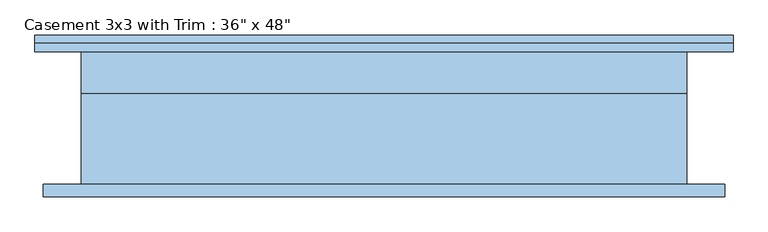
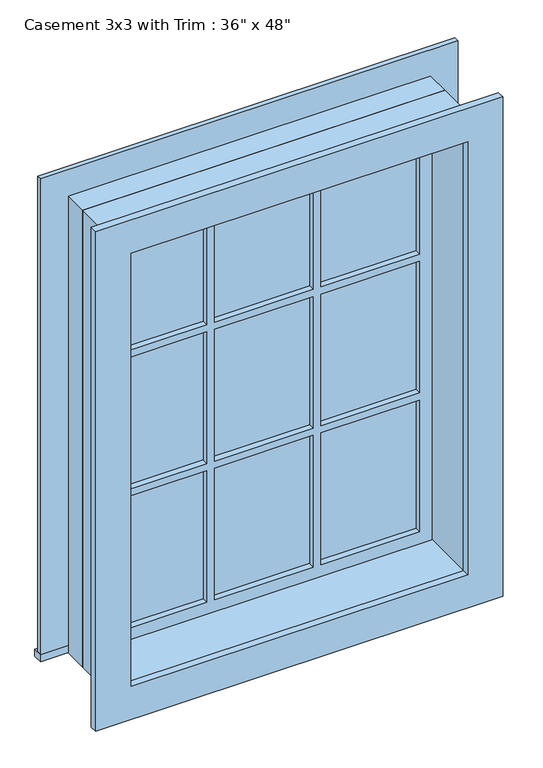
"""IFC4 building model written with IfcOpenShell, lengths in millimetres: window geometry."""

from ifc_helpers import new_model, si_unit, frame, origin, place, context, project, spatial, polyline, outline, extrude, source, transform, mapped, element, save


def window_ddc5d35f(model_context):
    return source(origin(), model_context, "Body", "SweptSolid", [
        extrude(outline(polyline([(-527.05, 125.4), (527.05, 125.4), (527.05, 100.0), (-527.05, 100.0), (-527.05, 125.4)])), frame((0.0, 0.0, 914.4), z_axis=(0.0, 0.0, 1.0), x_axis=(1.0, 0.0, 0.0)), (0.0, 0.0, 1.0), 19.05),
        extrude(outline(polyline([(2114.55, -438.15), (2114.55, 438.15), (933.45, 438.15), (933.45, 527.05), (2203.45, 527.05), (2203.45, -527.05), (933.45, -527.05), (933.45, -438.15), (2114.55, -438.15)])), frame((0.0, 100.0, 0.0), z_axis=(0.0, 1.0, 0.0), x_axis=(0.0, 0.0, 1.0)), (0.0, 0.0, 1.0), 12.7),
        extrude(outline(polyline([(143.9333333, 65.075), (393.7, 65.075), (393.7, 52.375), (143.9333333, 52.375), (143.9333333, 65.075)])), frame((0.0, 0.0, 1718.7333333), z_axis=(0.0, 0.0, 1.0), x_axis=(1.0, 0.0, 0.0)), (0.0, 0.0, 1.0), 351.3666667),
        extrude(outline(polyline([(-124.8833333, 65.075), (124.8833333, 65.075), (124.8833333, 52.375), (-124.8833333, 52.375), (-124.8833333, 65.075)])), frame((0.0, 0.0, 1718.7333333), z_axis=(0.0, 0.0, 1.0), x_axis=(1.0, 0.0, 0.0)), (0.0, 0.0, 1.0), 351.3666667),
        extrude(outline(polyline([(-393.7, 65.075), (-143.9333333, 65.075), (-143.9333333, 52.375), (-393.7, 52.375), (-393.7, 65.075)])), frame((0.0, 0.0, 1718.7333333), z_axis=(0.0, 0.0, 1.0), x_axis=(1.0, 0.0, 0.0)), (0.0, 0.0, 1.0), 351.3666667),
        extrude(outline(polyline([(-393.7, 65.075), (-143.9333333, 65.075), (-143.9333333, 52.375), (-393.7, 52.375), (-393.7, 65.075)])), frame((0.0, 0.0, 1348.3166667), z_axis=(0.0, 0.0, 1.0), x_axis=(1.0, 0.0, 0.0)), (0.0, 0.0, 1.0), 351.3666667),
        extrude(outline(polyline([(-124.8833333, 65.075), (124.8833333, 65.075), (124.8833333, 52.375), (-124.8833333, 52.375), (-124.8833333, 65.075)])), frame((0.0, 0.0, 1348.3166667), z_axis=(0.0, 0.0, 1.0), x_axis=(1.0, 0.0, 0.0)), (0.0, 0.0, 1.0), 351.3666667),
        extrude(outline(polyline([(143.9333333, 65.075), (393.7, 65.075), (393.7, 52.375), (143.9333333, 52.375), (143.9333333, 65.075)])), frame((0.0, 0.0, 1348.3166667), z_axis=(0.0, 0.0, 1.0), x_axis=(1.0, 0.0, 0.0)), (0.0, 0.0, 1.0), 351.3666667),
        extrude(outline(polyline([(143.9333333, 65.075), (393.7, 65.075), (393.7, 52.375), (143.9333333, 52.375), (143.9333333, 65.075)])), frame((0.0, 0.0, 977.9), z_axis=(0.0, 0.0, 1.0), x_axis=(1.0, 0.0, 0.0)), (0.0, 0.0, 1.0), 351.3666667),
        extrude(outline(polyline([(-124.8833333, 65.075), (124.8833333, 65.075), (124.8833333, 52.375), (-124.8833333, 52.375), (-124.8833333, 65.075)])), frame((0.0, 0.0, 977.9), z_axis=(0.0, 0.0, 1.0), x_axis=(1.0, 0.0, 0.0)), (0.0, 0.0, 1.0), 351.3666667),
        extrude(outline(polyline([(-393.7, 65.075), (-143.9333333, 65.075), (-143.9333333, 52.375), (-393.7, 52.375), (-393.7, 65.075)])), frame((0.0, 0.0, 977.9), z_axis=(0.0, 0.0, 1.0), x_axis=(1.0, 0.0, 0.0)), (0.0, 0.0, 1.0), 351.3666667),
        extrude(outline(polyline([(2190.75, 514.35), (2190.75, -514.35), (857.25, -514.35), (857.25, 514.35), (2190.75, 514.35)]), holes=[polyline([(2101.85, 425.45), (946.15, 425.45), (946.15, -425.45), (2101.85, -425.45), (2101.85, 425.45)])]), frame((0.0, -119.05, 0.0), z_axis=(0.0, 1.0, 0.0), x_axis=(0.0, 0.0, 1.0)), (0.0, 0.0, 1.0), 19.05),
        extrude(outline(polyline([(2114.55, -438.15), (933.45, -438.15), (933.45, 438.15), (2114.55, 438.15), (2114.55, -438.15)]), holes=[polyline([(2070.1, -143.9333333), (1718.7333333, -143.9333333), (1718.7333333, -393.7), (2070.1, -393.7), (2070.1, -143.9333333)]), polyline([(1699.6833333, -143.9333333), (1348.3166667, -143.9333333), (1348.3166667, -393.7), (1699.6833333, -393.7), (1699.6833333, -143.9333333)]), polyline([(1329.2666667, -143.9333333), (977.9, -143.9333333), (977.9, -393.7), (1329.2666667, -393.7), (1329.2666667, -143.9333333)]), polyline([(2070.1, 124.8833333), (1718.7333333, 124.8833333), (1718.7333333, -124.8833333), (2070.1, -124.8833333), (2070.1, 124.8833333)]), polyline([(1699.6833333, 124.8833333), (1348.3166667, 124.8833333), (1348.3166667, -124.8833333), (1699.6833333, -124.8833333), (1699.6833333, 124.8833333)]), polyline([(1329.2666667, 124.8833333), (977.9, 124.8833333), (977.9, -124.8833333), (1329.2666667, -124.8833333), (1329.2666667, 124.8833333)]), polyline([(2070.1, 393.7), (1718.7333333, 393.7), (1718.7333333, 143.9333333), (2070.1, 143.9333333), (2070.1, 393.7)]), polyline([(1699.6833333, 393.7), (1348.3166667, 393.7), (1348.3166667, 143.9333333), (1699.6833333, 143.9333333), (1699.6833333, 393.7)]), polyline([(1329.2666667, 393.7), (977.9, 393.7), (977.9, 143.9333333), (1329.2666667, 143.9333333), (1329.2666667, 393.7)])]), frame((0.0, 36.5, 0.0), z_axis=(0.0, 1.0, 0.0), x_axis=(0.0, 0.0, 1.0)), (0.0, 0.0, 1.0), 44.45),
        extrude(outline(polyline([(2133.6, -457.2), (914.4, -457.2), (914.4, 457.2), (2133.6, 457.2), (2133.6, -457.2)]), holes=[polyline([(2101.85, -425.45), (2101.85, 425.45), (946.15, 425.45), (946.15, -425.45), (2101.85, -425.45)])]), frame((0.0, -100.0, 0.0), z_axis=(0.0, 1.0, 0.0), x_axis=(0.0, 0.0, 1.0)), (0.0, 0.0, 1.0), 136.5),
        extrude(outline(polyline([(2133.6, 457.2), (2133.6, -457.2), (914.4, -457.2), (914.4, 457.2), (2133.6, 457.2)]), holes=[polyline([(2114.55, 438.15), (933.45, 438.15), (933.45, -438.15), (2114.55, -438.15), (2114.55, 438.15)])]), frame((0.0, 36.5, 0.0), z_axis=(0.0, 1.0, 0.0), x_axis=(0.0, 0.0, 1.0)), (0.0, 0.0, 1.0), 63.5),
    ])


if __name__ == "__main__":
    model = new_model("IFC4")
    model_context = context("Model", 3, world=origin())
    ifc_project = project(units=[si_unit("LENGTHUNIT", "METRE", prefix="MILLI")], contexts=[model_context])
    site = spatial("IfcSite", under=ifc_project)
    building = spatial("IfcBuilding", under=site)
    placement = place(None, origin())
    window_shape = window_ddc5d35f(model_context)
    element("IfcWindow", 1, ObjectType="Casement 3x3 with Trim : 36\" x 48\"", at=placement, inside=building, context=model_context, shape_type="MappedRepresentation", body=[
        mapped(window_shape, transform((0.0, 0.0, 0.0), x_axis=(1.0, 0.0, 0.0), y_axis=(0.0, 1.0, 0.0), z_axis=(0.0, 0.0, 1.0))),
    ])
    save(model, "model.ifc")

# Revit data of these elements
# Type "Casement 3x3 with Trim : 36\" x 48\""
#   Type Mark = "19"
#   Construction Type Id = "GSP4R"
#   Assembly Code = "B2020100"
#   Analytic Construction = "1/8 in Pilkington single glazing"
#   Visual Light Transmittance = 0.9
#   Solar Heat Gain Coefficient = 0.78
#   Heat Transfer Coefficient (U) = 3.6886 W/(m²·K)
#   Height = 4' - 0"
#   Default Sill Height = 3' - 0"
#   Trim Projection - Ext. = 0' - 0 1/2"
#   Trim Projection - Int. = 0' - 0 3/4"
#   Trim Width - Exterior = 0' - 3 1/2"
#   Trim Width - Interior = 0' - 3 1/2"
#   Width = 3' - 0"
#   Window Inset = 0' - 0 3/4"
#   Define Thermal Properties by = 1
#   Glass Pane Material = Glass
#   Sash Material = Sash
#   Trim Exterior Material = Trim
#   Trim Interior Material = Trim
#   Wall Closure = (empty or 0)
# Element 1 (IfcWindow, "Casement 3x3 with Trim : 36\" x 48\"")
#   Materials on its faces: "Sash", "Glass", "Trim"
# Materials
#   "Glass": class "Glass", colour RGB 218 227 224, transparency 0.85, Description = "Soda Lime Glass", Cost = 0
#   "Sash": class "Wood", colour RGB 136 99 55, transparency 0
#   "Trim": class "Wood", colour RGB 224 178 126, transparency 0
